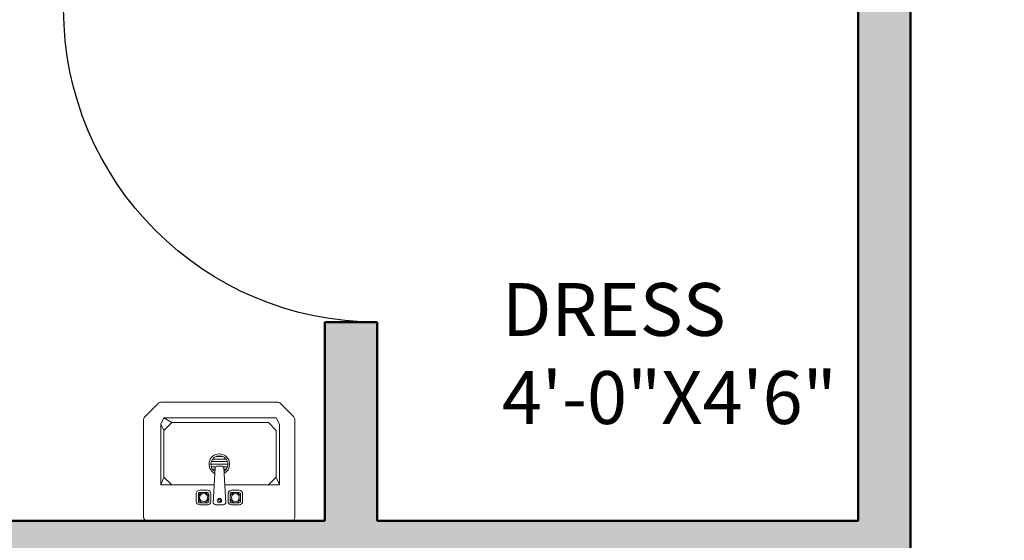
# Model space of a CAD drawing. Units: inches. Extents: x -7 to 1228, y -146 to 1091.
# Tile 74 of 88: x 722 to 816, y 785 to 835. Entities that reach past the tile are written whole.
import ezdxf

# ---------------------------------------------------------------- set-up
doc = ezdxf.new("R2010")
doc.units = ezdxf.units.IN
for name, color, linetype, lineweight in [('A-AREA-IDEN', 7, 'Continuous', 18), ('A-DOOR', 4, 'Continuous', 25), ('A-FURN', 8, 'Continuous', 18), ('A-WALL', 7, 'Continuous', 50), ('A-WALL-PATT', 251, 'Continuous', 13)]:
    doc.layers.add(name, color=color, linetype=linetype, lineweight=lineweight)
doc.styles.get("Standard").update_dxf_attribs({"font": 'arial.ttf'})

# ---------------------------------------------------------------- blocks, each defined once
blk = doc.blocks.new('A$C4CB854FF')
for p, q in [((0.4725, 0.38), (0.0125, 0.38)), ((0, 0.3675), (0, 0.0552)), ((0.485, 0.0552), (0.485, 0.3675)), ((0.1677, 0.2932), (0.1677, 0.318)), ((0.1745, 0.2919), (0.1745, 0.3194)), ((0.1773, 0.3221), (0.2048, 0.3221)), ((0.1787, 0.329), (0.2034, 0.329)), ((0.2075, 0.3194), (0.2075, 0.2919)), ((0.2144, 0.318), (0.2144, 0.2932)), ((0.2279, 0.2104), (0.2213, 0.3235)), ((0.2337, 0.329), (0.2502, 0.329)), ((0.2625, 0.3235), (0.256, 0.2104)), ((0.2694, 0.318), (0.2694, 0.2932)), ((0.2763, 0.3194), (0.2763, 0.2919)), ((0.3065, 0.3221), (0.279, 0.3221)), ((0.3052, 0.329), (0.2804, 0.329)), ((0.3093, 0.2919), (0.3093, 0.3194)), ((0.3162, 0.2932), (0.3162, 0.318)), ((0.2048, 0.2891), (0.1773, 0.2891)), ((0.279, 0.2891), (0.3065, 0.2891)), ((0.05, 0.265), (0.2247, 0.265)), ((0.06, 0.24), (0.05, 0.265)), ((0.05, 0.07), (0.05, 0.265)), ((0.085, 0.265), (0.06, 0.24)), ((0.2034, 0.2822), (0.1787, 0.2822)), ((0.2591, 0.265), (0.43, 0.265)), ((0.2804, 0.2822), (0.3052, 0.2822)), ((0.395, 0.265), (0.42, 0.24)), ((0.42, 0.24), (0.43, 0.265)), ((0.43, 0.07), (0.43, 0.265)), ((0.06, 0.24), (0.06, 0.09)), ((0.42, 0.24), (0.42, 0.09)), ((0.2152, 0.1984), (0.2694, 0.1984)), ((0.2297, 0.2066), (0.2165, 0.2066)), ((0.2681, 0.1901), (0.2165, 0.1901)), ((0.2272, 0.2149), (0.2208, 0.2149)), ((0.2505, 0.2052), (0.2334, 0.2052)), ((0.2681, 0.2066), (0.2541, 0.2066)), ((0.2638, 0.2149), (0.2566, 0.2149)), ((0.2638, 0.1819), (0.2208, 0.1819)), ((0.2533, 0.1736), (0.2313, 0.1736)), ((0.05, 0.07), (0.06, 0.05)), ((0.06, 0.09), (0.085, 0.065)), ((0.085, 0.065), (0.395, 0.065)), ((0.42, 0.09), (0.395, 0.065)), ((0.395, 0.065), (0.42, 0.05)), ((0.42, 0.09), (0.43, 0.07)), ((0.43, 0.07), (0.42, 0.05)), ((0.0037, 0.0463), (0.0463, 0.0037)), ((0.42, 0.05), (0.06, 0.05)), ((0.4387, 0.0037), (0.4813, 0.0463)), ((0.0552, 0), (0.4298, 0))]:
    blk.add_line(p, q)
for centre, radius in [((0.191, 0.3056), 0.0165), ((0.191, 0.3056), 0.0127), ((0.2419, 0.3152), 0.00688), ((0.2419, 0.3152), 0.00344), ((0.2928, 0.3056), 0.0165), ((0.2928, 0.3056), 0.0127)]:
    blk.add_circle(centre, radius)
for centre, radius, start, end in [((0.0125, 0.3675), 0.0125, 90, 180), ((0.4725, 0.3675), 0.0125, 0, 90), ((0.1787, 0.318), 0.011, 90, 180), ((0.1773, 0.3194), 0.00275, 90, 180), ((0.2034, 0.318), 0.011, 0, 90), ((0.2048, 0.3194), 0.00275, 360, 90), ((0.2329, 0.314), 0.015, 87.1975, 140.7274), ((0.2509, 0.314), 0.015, 39.2726, 92.8025), ((0.2804, 0.318), 0.011, 90, 180), ((0.279, 0.3194), 0.00275, 90, 180), ((0.3052, 0.318), 0.011, 0, 90), ((0.3065, 0.3194), 0.00275, 360, 90), ((0.1787, 0.2932), 0.011, 180, 270), ((0.1773, 0.2919), 0.00275, 180, 270), ((0.2034, 0.2932), 0.011, 270, 0), ((0.2048, 0.2919), 0.00275, 270, 0), ((0.2804, 0.2932), 0.011, 180, 270), ((0.279, 0.2919), 0.00275, 180, 270), ((0.3052, 0.2932), 0.011, 270, 360), ((0.3065, 0.2919), 0.00275, 270, 0), ((0.2423, 0.1984), 0.033, 118.6883, 62.8686), ((0.2423, 0.1984), 0.0271, 124.7758, 57.2247), ((0.2334, 0.2107), 0.0055, 183.3274, 270), ((0.2505, 0.2107), 0.0055, 270, 356.6726), ((0.0125, 0.0552), 0.0125, 180, 225), ((0.4725, 0.0552), 0.0125, 315, 0), ((0.0552, 0.0125), 0.0125, 225, 270), ((0.4298, 0.0125), 0.0125, 270, 315)]:
    blk.add_arc(centre, radius, start, end)
blk = doc.blocks.new('DOOR-750')
blk.add_line((30, 30), (30, 0))
blk.add_arc((30, 30), 30, 180, 270)

msp = doc.modelspace()

# ---------------------------------------------------------------- hatches: boundary and pattern name
at = {"layer": 'A-WALL-PATT'}
h = msp.add_hatch(color=256, dxfattribs=at)
h.dxf.hatch_style = 1
h.paths.add_polyline_path([(69, 568), (60, 568), (60, 493), (63.289, 493), (69, 493)])
h.paths.add_polyline_path([(69, 662.405), (60, 662.405), (60, 586), (69, 586)], flags=17)
h.paths.add_polyline_path([(69, 723), (184, 723), (184, 734), (179, 734), (179, 728), (69, 728), (69, 741.623), (60, 741.623), (60, 698.405), (69, 698.405)], flags=17)
h.paths.add_polyline_path([(69, 782), (231, 782), (231, 728), (231, 723), (231, 586), (236, 586), (236, 787), (69, 787), (69, 800.126), (60, 800.126), (60, 765.623), (69, 765.623)])
h.paths.add_polyline_path([(184, 842), (189, 842), (189, 848), (173, 848), (173, 842), (179, 842), (179, 787), (184, 787)])
h.paths.add_polyline_path([(118.22, 69), (69, 69), (69, 60), (118.22, 60)])
h.paths.add_polyline_path([(227, 69), (154.22, 69), (154.22, 60), (227, 60)])
h.paths.add_polyline_path([(236, 60), (232.711, 60), (227, 60), (227, 36), (236, 36)])
h.paths.add_polyline_path([(389, 60), (380, 60), (380, 36), (389, 36)])
h.paths.add_polyline_path([(384, 181), (380, 181), (380, 115), (380, 78), (384, 78)])
h.paths.add_polyline_path([(380, 115), (334.547, 115), (334.547, 109), (380, 109)])
h.paths.add_polyline_path([(274.547, 115), (236, 115), (236, 201), (232.711, 201), (231, 201), (231, 78), (236, 78), (236, 109), (274.547, 109)])
h.paths.add_polyline_path([(69, 123), (60, 123), (60, 78), (69, 78)])
h.paths.add_polyline_path([(69, 201), (60, 201), (60, 159), (69, 159)])
h.paths.add_polyline_path([(143, 219), (69, 219), (69, 213), (143, 213)], flags=17)
h.paths.add_polyline_path([(189, 219), (184, 219), (184, 274), (231, 274), (231, 219), (236, 219), (236, 279), (184, 279), (184, 297), (179, 297), (179, 279), (69, 279), (69, 290.912), (60, 290.912), (60, 262.179), (69, 262.179), (69, 274), (179, 274), (179, 219), (173, 219), (173, 213), (189, 213)])
h.paths.add_polyline_path([(69, 238.179), (60, 238.179), (60, 219), (69, 219)], flags=17)
h.paths.add_polyline_path([(69, 333), (60, 333), (60, 314.912), (69, 314.912), (69, 316.965)])
h.paths.add_polyline_path([(190, 338), (184, 338), (69, 338), (69, 333), (179, 333), (179, 327), (184, 327), (184, 333.021), (190, 333.046)])
h.paths.add_polyline_path([(69, 386.806), (60, 386.806), (60, 351), (69, 351)])
h.paths.add_polyline_path([(69, 475), (60, 475), (60, 422.806), (69, 422.806)])
h.paths.add_polyline_path([(236, 475), (231, 475), (231, 351.238), (236, 351.238)])
h.paths.add_polyline_path([(384, 475), (380, 475), (380, 362), (384, 362)])
h.paths.add_polyline_path([(547, 307), (439, 307), (439, 356), (445, 356), (445, 362), (433, 362), (433, 307), (380, 307), (380, 244), (380, 241), (384, 241), (384, 301), (433, 301), (433, 277), (439, 277), (439, 301), (547, 301)])
h.paths.add_polyline_path([(547, 241), (439, 241), (439, 247), (433, 247), (433, 235), (547, 235)])
h.paths.add_polyline_path([(450, 69), (440.286, 69), (424.889, 69), (389, 69), (389, 60), (450, 60)])
h.paths.add_polyline_path([(547, 69), (486, 69), (486, 60), (547, 60)])
h.paths.add_polyline_path([(556, 148.268), (547, 148.268), (547, 78), (556, 78)])
h.paths.add_polyline_path([(556, 223), (547, 223), (547, 195), (547, 184.268), (556, 184.268)])
h.paths.add_polyline_path([(556, 311.192), (547, 311.192), (547, 273.075), (556, 273.075)])
h.paths.add_polyline_path([(556, 344), (552.711, 344), (547, 344), (547, 335.192), (556, 335.192)])
h.paths.add_polyline_path([(556, 249.075), (547, 249.075), (547, 241), (556, 241)])
h.paths.add_polyline_path([(547, 362), (475, 362), (475, 356), (547, 356)], flags=0)
h.paths.add_polyline_path([(556, 399.621), (547, 399.621), (547, 362), (556, 362)])
h.paths.add_polyline_path([(556, 475), (547, 475), (547, 435.621), (556, 435.621)])
h.paths.add_polyline_path([(547, 493), (389, 493), (389, 487), (547, 487)])
h.paths.add_polyline_path([(380, 493), (278, 493), (278, 487), (380, 487)])
h.paths.add_polyline_path([(227, 493), (69, 493), (69, 487), (227, 487)])
h.paths.add_polyline_path([(643, 122.445), (634, 122.445), (634, 78), (643, 78)])
h.paths.add_polyline_path([(702.5, 69), (692.786, 69), (677.389, 69), (643, 69), (643, 60), (702.5, 60)])
h.paths.add_polyline_path([(798, 69), (738.5, 69), (738.5, 60), (798, 60)])
h.paths.add_polyline_path([(807, 60), (803.711, 60), (798, 60), (798, 36), (807, 36)])
h.paths.add_polyline_path([(807, 109), (846.751, 109), (846.751, 115), (807, 115), (807, 159), (802, 159), (802, 78), (807, 78)])
h.paths.add_polyline_path([(807, 201), (802, 201), (802, 195), (807, 195)])
h.paths.add_polyline_path([(643, 201), (634, 201), (634, 158.445), (643, 158.445)])
h.paths.add_polyline_path([(756, 225), (751, 225), (751, 219), (643, 219), (643, 213), (756, 213)])
h.paths.add_polyline_path([(643, 240.848), (634, 240.848), (634, 219), (643, 219)])
h.paths.add_polyline_path([(643, 274), (643, 288.629), (634, 288.629), (634, 264.848), (643, 264.848)])
h.paths.add_polyline_path([(802, 279), (756, 279), (756, 297), (751, 297), (751, 279), (643, 279), (643, 274), (751, 274), (751, 255), (756, 255), (756, 274), (802, 274)])
h.paths.add_polyline_path([(807, 333), (803.711, 333), (802, 333), (802, 279), (802, 274), (802, 219), (807, 219)])
h.paths.add_polyline_path([(956, 182), (951, 182), (951, 115), (906.751, 115), (906.751, 109), (951, 109), (951, 78), (956, 78)])
h.paths.add_polyline_path([(960, 60), (951, 60), (951, 36), (960, 36)])
h.paths.add_polyline_path([(1021, 69), (1005.781, 69), (960, 69), (960, 60), (1021, 60)])
h.paths.add_polyline_path([(956, 224), (951, 224), (951, 218), (956, 218)])
h.paths.add_polyline_path([(956, 302), (1004, 302), (1004, 278), (1010, 278), (1010, 302), (1118, 302), (1118, 290.809), (1127, 290.809), (1127, 326.968), (1118, 326.968), (1118, 320.966), (1118, 307), (1010, 307), (1010, 356), (1016, 356), (1016, 362), (1004, 362), (1004, 307), (951, 307), (951, 244), (951, 242), (954.289, 242), (956, 242)])
h.paths.add_polyline_path([(643, 333), (634, 333), (634, 312.629), (643, 312.629), (643, 316.965)])
h.paths.add_polyline_path([(756, 338), (643, 338), (643, 333), (751, 333), (751, 327), (756, 327)])
h.paths.add_polyline_path([(643, 388), (634, 388), (634, 351), (643, 351)])
h.paths.add_polyline_path([(807, 357), (802, 357), (802, 351), (807, 351)])
h.paths.add_polyline_path([(807, 475), (802, 475), (802, 393), (807, 393)])
h.paths.add_polyline_path([(643, 475), (634, 475), (634, 424), (643, 424)])
h.paths.add_polyline_path([(798, 493), (643, 493), (643, 487), (798, 487)])
h.paths.add_polyline_path([(634, 493), (556, 493), (556, 487), (634, 487)])
h.paths.add_polyline_path([(813, 493), (807, 493), (807, 487), (813, 487)])
h.paths.add_polyline_path([(951, 493), (849, 493), (849, 487), (951, 487)])
h.paths.add_polyline_path([(956, 484), (951, 484), (951, 374), (956, 374)])
h.paths.add_polyline_path([(1109, 493), (969, 493), (969, 487), (1109, 487)])
h.paths.add_polyline_path([(1127, 484), (1118, 484), (1118, 450.641), (1127, 450.641)])
h.paths.add_polyline_path([(1127, 414.641), (1118, 414.641), (1118, 365), (1127, 365)])
h.paths.add_polyline_path([(1109, 362), (1046, 362), (1046, 356), (1109, 356)], flags=17)
h.paths.add_polyline_path([(1127, 356), (1123.454, 356), (1118, 356), (1118, 350.968), (1127, 350.968)], flags=0)
h.paths.add_polyline_path([(1127, 266.809), (1118, 266.809), (1118, 262.361), (1118, 242), (1127, 242)], flags=17)
h.paths.add_polyline_path([(1118, 242), (1010, 242), (1010, 248), (1004, 248), (1004, 237), (1118, 237)])
h.paths.add_polyline_path([(1127, 224), (1118, 224), (1118, 170), (1127, 170)])
h.paths.add_polyline_path([(1127, 134), (1118, 134), (1118, 78), (1127, 78)])
h.paths.add_polyline_path([(1118, 69), (1057, 69), (1057, 60), (1118, 60)])
h.paths.add_polyline_path([(227, 571.546), (227, 574), (69, 574), (69, 568), (227, 568)])
h.paths.add_polyline_path([(380, 571.546), (380, 574), (278, 574), (278, 568), (380, 568)])
h.paths.add_polyline_path([(242, 574), (236, 574), (236, 568), (242, 568)])
h.paths.add_polyline_path([(547, 571.546), (547, 574), (389, 574), (389, 568), (547, 568)])
h.paths.add_polyline_path([(384, 733), (380, 733), (380, 586), (384, 586)])
h.paths.add_polyline_path([(556, 646), (634, 646), (634, 655), (547, 655), (547, 586), (556, 586)])
h.paths.add_polyline_path([(634, 574), (556, 574), (556, 568), (634, 568)])
h.paths.add_polyline_path([(643, 655), (634, 655), (634, 586), (643, 586)])
h.paths.add_polyline_path([(798, 574), (643, 574), (643, 568), (798, 568)])
h.paths.add_polyline_path([(643, 663.854), (634, 663.854), (634, 655), (643, 655)])
h.paths.add_polyline_path([(556, 676.967), (547, 676.967), (547, 655), (556, 655)])
h.paths.add_polyline_path([(556, 733), (547, 733), (547, 712.967), (556, 712.967)])
h.paths.add_polyline_path([(643, 710), (634, 710), (634, 699.854), (643, 699.854)])
h.paths.add_polyline_path([(807, 668), (802, 668), (802, 586), (807, 586)])
h.paths.add_polyline_path([(951, 574), (849, 574), (849, 568), (951, 568)])
h.paths.add_polyline_path([(956, 691), (951, 691), (951, 577), (956, 577)])
h.paths.add_polyline_path([(1109, 574), (969, 574), (969, 568), (1109, 568)])
h.paths.add_polyline_path([(1127, 643.403), (1118, 643.403), (1118, 577), (1127, 577)])
h.paths.add_polyline_path([(1127, 568), (1123.454, 568), (1118, 568), (1118, 493), (1127, 493)])
h.paths.add_polyline_path([(1127, 733), (1118, 733), (1118, 679.403), (1127, 679.403)])
h.paths.add_polyline_path([(1127, 777.348), (1118, 777.348), (1118, 770.035), (1118, 751), (1127, 751)], flags=17)
h.paths.add_polyline_path([(1118, 751), (1010, 751), (1010, 757), (1004, 757), (1004, 745), (1118, 745)])
h.paths.add_polyline_path([(956, 811), (1004, 811), (1004, 787), (1010, 787), (1010, 811), (1017.874, 811), (1017.874, 811.627, -0.414214), (1018.247, 812), (1031.978, 812, -0.414214), (1032.351, 811.627), (1032.351, 811), (1118, 811), (1118, 801.348), (1127, 801.348), (1127, 834.685), (1118, 834.685), (1118, 830.238), (1118, 817), (1010, 817), (1010, 866), (1016, 866), (1016, 872), (1004, 872), (1004, 817), (956, 817), (956, 866), (951, 866), (951, 751), (954.289, 751), (956, 751)])
h.paths.add_polyline_path([(1118, 872), (1046, 872), (1046, 866), (1118, 866)], flags=17)
h.paths.add_polyline_path([(1127, 924.711), (1118, 924.711), (1118, 884), (1127, 884)])
h.paths.add_polyline_path([(1127, 866), (1123.711, 866), (1118, 866), (1118, 858.685), (1127, 858.685)], flags=17)
h.paths.add_polyline_path([(956, 983), (951, 983), (951, 952), (807, 952), (807, 983), (802, 983), (802, 902), (807, 902), (807, 946), (951, 946), (951, 884), (956, 884)])
h.paths.add_polyline_path([(807, 842), (802, 842), (802, 787), (756, 787), (756, 806), (751, 806), (751, 787), (643, 787), (643, 782), (751, 782), (751, 764), (756, 764), (756, 782), (802, 782), (802, 728), (807, 728)])
h.paths.add_polyline_path([(756, 848), (643, 848), (643, 842), (751, 842), (751, 836), (756, 836)])
h.paths.add_polyline_path([(756, 734), (751, 734), (751, 728), (643, 728), (643, 723), (756, 723)])
h.paths.add_polyline_path([(643, 749.791), (634, 749.791), (634, 728), (637.289, 728), (643, 728)])
h.paths.add_polyline_path([(643, 805.405), (634, 805.405), (634, 773.791), (643, 773.791)])
h.paths.add_polyline_path([(643, 896.663), (634, 896.663), (634, 860), (637.289, 860), (643, 860)])
h.paths.add_polyline_path([(643, 842), (634, 842), (634, 829.405), (643, 829.405)])
h.paths.add_polyline_path([(643, 983), (634, 983), (634, 932.663), (643, 932.663)])
h.paths.add_polyline_path([(1127, 983), (1118, 983), (1118, 960.711), (1127, 960.711)])
h.paths.add_polyline_path([(1118, 1001), (1077.525, 1001), (1077.525, 992), (1118, 992)])
h.paths.add_polyline_path([(1041.525, 1001), (960, 1001), (960, 992), (1041.525, 992)])
h.paths.add_polyline_path([(960, 1025), (951, 1025), (951, 1001), (954.289, 1001), (960, 1001)])
h.paths.add_polyline_path([(807, 1025), (798, 1025), (798, 1001), (807, 1001)])
h.paths.add_polyline_path([(798, 1001), (738.5, 1001), (738.5, 992), (798, 992)])
h.paths.add_polyline_path([(702.5, 1001), (643, 1001), (643, 992), (702.5, 992)])
h.paths.add_polyline_path([(547, 1001), (499.113, 1001), (499.113, 992), (547, 992)])
h.paths.add_polyline_path([(463.113, 1001), (389, 1001), (389, 992), (463.113, 992)])
h.paths.add_polyline_path([(389, 1025), (380, 1025), (380, 1022), (380, 1001), (383.289, 1001), (389, 1001)])
h.paths.add_polyline_path([(236, 1025), (227, 1025), (227, 1001), (236, 1001)])
h.paths.add_polyline_path([(236, 983), (231, 983), (231, 860), (236, 860)])
h.paths.add_polyline_path([(274.547, 952), (236, 952), (236, 946), (274.547, 946)])
h.paths.add_polyline_path([(380, 952), (334.547, 952), (334.547, 946), (380, 946)])
h.paths.add_polyline_path([(384, 983), (380, 983), (380, 884), (383.289, 884), (384, 884)])
h.paths.add_polyline_path([(227, 1001), (155.012, 1001), (155.012, 992), (162.875, 992), (227, 992)])
h.paths.add_polyline_path([(119.012, 1001), (69, 1001), (69, 992), (119.012, 992)])
h.paths.add_polyline_path([(69, 983), (60, 983), (60, 922.987), (69, 922.987)])
h.paths.add_polyline_path([(69, 886.987), (60, 886.987), (60, 860), (63.289, 860), (69, 860)])
h.paths.add_polyline_path([(143, 848), (69, 848), (69, 842), (143, 842)])

# ---------------------------------------------------------------- linework, layer by layer
at = {"layer": 'A-WALL'}
for p, q in [((802, 787), (802, 866)), ((807, 866), (807, 704)), ((807, 704), (807, 866)), ((802, 842), (802, 787)), ((756, 806), (751, 806)), ((751, 806), (751, 787)), ((756, 806), (756, 787)), ((751, 787), (643, 787)), ((802, 787), (756, 787))]:
    msp.add_line(p, q, dxfattribs=at)

# ---------------------------------------------------------------- block references
at = {"layer": 'A-DOOR', "extrusion": (0, 0, -1), "zscale": -1, "rotation": 90}
msp.add_blockref('DOOR-750', (-726, 806), dxfattribs=at)
at = {"layer": 'A-FURN', "xscale": 29.84864686937646, "yscale": 29.84864686937646, "zscale": 29.84864686937646, "rotation": 180}
msp.add_blockref('A$C4CB854FF', (748.128, 798.342), dxfattribs=at)

# ---------------------------------------------------------------- texts
at = {"layer": 'A-AREA-IDEN', "insert": (767.923, 809.755), "char_height": 5.0568, "attachment_point": 1}
msp.add_mtext_dynamic_manual_height_columns('DRESS\\P4\'-0"X4\'6"', width=137.28212, gutter_width=25.284, heights=[0], dxfattribs=at)

doc.saveas('drawing.dxf')
